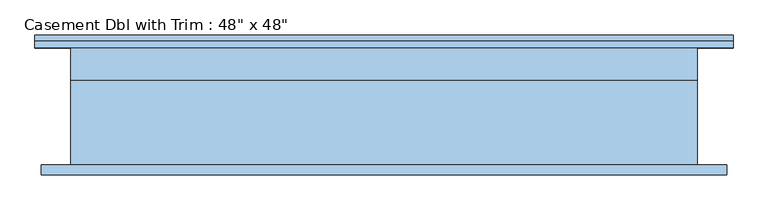
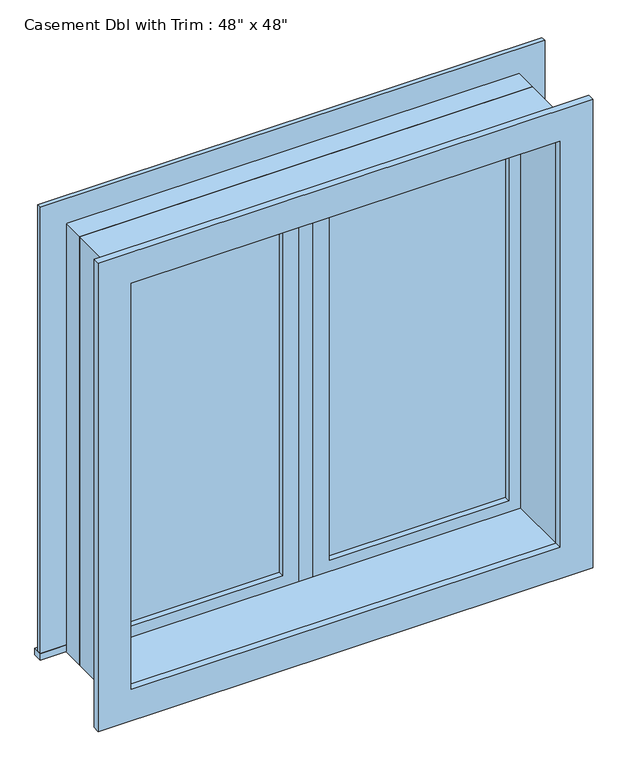
"""IFC4 building model written with IfcOpenShell, lengths in millimetres: window geometry."""

from ifc_helpers import new_model, si_unit, frame, origin, place, context, project, spatial, polyline, outline, extrude, source, transform, mapped, element, save


def window_534dcd48(model_context):
    return source(origin(), model_context, "Body", "SweptSolid", [
        extrude(outline(polyline([(63.5, 98.425), (546.1, 98.425), (546.1, 85.725), (63.5, 85.725), (63.5, 98.425)])), frame((0.0, 0.0, 977.9), z_axis=(0.0, 0.0, 1.0), x_axis=(1.0, 0.0, 0.0)), (0.0, 0.0, 1.0), 1092.2),
        extrude(outline(polyline([(2114.55, 19.05), (933.45, 19.05), (933.45, 590.55), (2114.55, 590.55), (2114.55, 19.05)]), holes=[polyline([(2070.1, 63.5), (2070.1, 546.1), (977.9, 546.1), (977.9, 63.5), (2070.1, 63.5)])]), frame((0.0, 69.85, 0.0), z_axis=(0.0, 1.0, 0.0), x_axis=(0.0, 0.0, 1.0)), (0.0, 0.0, 1.0), 44.45),
        extrude(outline(polyline([(19.05, 69.85), (-19.05, 69.85), (-19.05, 133.35), (19.05, 133.35), (19.05, 69.85)])), frame((0.0, 0.0, 933.45), z_axis=(0.0, 0.0, 1.0), x_axis=(1.0, 0.0, 0.0)), (0.0, 0.0, 1.0), 1181.1),
        extrude(outline(polyline([(-679.45, 158.75), (679.45, 158.75), (679.45, 133.35), (-679.45, 133.35), (-679.45, 158.75)])), frame((0.0, 0.0, 914.4), z_axis=(0.0, 0.0, 1.0), x_axis=(1.0, 0.0, 0.0)), (0.0, 0.0, 1.0), 19.05),
        extrude(outline(polyline([(2114.55, -590.55), (2114.55, 590.55), (933.45, 590.55), (933.45, 679.45), (2203.45, 679.45), (2203.45, -679.45), (933.45, -679.45), (933.45, -590.55), (2114.55, -590.55)])), frame((0.0, 133.35, 0.0), z_axis=(0.0, 1.0, 0.0), x_axis=(0.0, 0.0, 1.0)), (0.0, 0.0, 1.0), 12.7),
        extrude(outline(polyline([(2190.75, 666.75), (2190.75, -666.75), (857.25, -666.75), (857.25, 666.75), (2190.75, 666.75)]), holes=[polyline([(2101.85, 577.85), (946.15, 577.85), (946.15, -577.85), (2101.85, -577.85), (2101.85, 577.85)])]), frame((0.0, -114.3, 0.0), z_axis=(0.0, 1.0, 0.0), x_axis=(0.0, 0.0, 1.0)), (0.0, 0.0, 1.0), 19.05),
        extrude(outline(polyline([(-63.5, 85.725), (-546.1, 85.725), (-546.1, 98.425), (-63.5, 98.425), (-63.5, 85.725)])), frame((0.0, 0.0, 977.9), z_axis=(0.0, 0.0, 1.0), x_axis=(1.0, 0.0, 0.0)), (0.0, 0.0, 1.0), 1092.2),
        extrude(outline(polyline([(2114.55, -590.55), (933.45, -590.55), (933.45, -19.05), (2114.55, -19.05), (2114.55, -590.55)]), holes=[polyline([(2070.1, -546.1), (2070.1, -63.5), (977.9, -63.5), (977.9, -546.1), (2070.1, -546.1)])]), frame((0.0, 69.85, 0.0), z_axis=(0.0, 1.0, 0.0), x_axis=(0.0, 0.0, 1.0)), (0.0, 0.0, 1.0), 44.45),
        extrude(outline(polyline([(2133.6, -609.6), (914.4, -609.6), (914.4, 609.6), (2133.6, 609.6), (2133.6, -609.6)]), holes=[polyline([(2101.85, -577.85), (2101.85, 577.85), (946.15, 577.85), (946.15, -577.85), (2101.85, -577.85)])]), frame((0.0, -95.25, 0.0), z_axis=(0.0, 1.0, 0.0), x_axis=(0.0, 0.0, 1.0)), (0.0, 0.0, 1.0), 165.1),
        extrude(outline(polyline([(2133.6, 609.6), (2133.6, -609.6), (914.4, -609.6), (914.4, 609.6), (2133.6, 609.6)]), holes=[polyline([(2114.55, 590.55), (933.45, 590.55), (933.45, -590.55), (2114.55, -590.55), (2114.55, 590.55)])]), frame((0.0, 69.85, 0.0), z_axis=(0.0, 1.0, 0.0), x_axis=(0.0, 0.0, 1.0)), (0.0, 0.0, 1.0), 63.5),
    ])


if __name__ == "__main__":
    model = new_model("IFC4")
    model_context = context("Model", 3, world=origin())
    ifc_project = project(units=[si_unit("LENGTHUNIT", "METRE", prefix="MILLI")], contexts=[model_context])
    site = spatial("IfcSite", under=ifc_project)
    building = spatial("IfcBuilding", under=site)
    placement = place(None, origin())
    window_shape = window_534dcd48(model_context)
    element("IfcWindow", 1, ObjectType="Casement Dbl with Trim : 48\" x 48\"", at=placement, inside=building, context=model_context, shape_type="MappedRepresentation", body=[
        mapped(window_shape, transform((0.0, 0.0, 0.0), x_axis=(1.0, 0.0, 0.0), y_axis=(0.0, 1.0, 0.0), z_axis=(0.0, 0.0, 1.0))),
    ])
    save(model, "model.ifc")

# Revit data of these elements
# Type "Casement Dbl with Trim : 48\" x 48\""
#   Type Mark = "19"
#   Construction Type Id = "GSP4R"
#   Assembly Code = "B2020100"
#   Analytic Construction = "1/8 in Pilkington single glazing"
#   Visual Light Transmittance = 0.9
#   Solar Heat Gain Coefficient = 0.78
#   Heat Transfer Coefficient (U) = 0.6496 BTU/(h·ft²·°F)
#   Height = 4' - 0"
#   Default Sill Height = 3' - 0"
#   Trim Projection - Ext. = 0' - 0 1/2"
#   Trim Projection - Int. = 0' - 0 3/4"
#   Trim Width - Exterior = 0' - 3 1/2"
#   Trim Width - Interior = 0' - 3 1/2"
#   Width = 4' - 0"
#   Window Inset = 0' - 0 3/4"
#   Define Thermal Properties by = 1
#   Glass Pane Material = Glass
#   Sash Material = Sash
#   Trim Exterior Material = Trim
#   Trim Interior Material = Trim
#   Wall Closure = (empty or 0)
# Element 1 (IfcWindow, "Casement Dbl with Trim : 48\" x 48\"")
#   Materials on its faces: "Sash", "Trim", "Glass"
# Materials
#   "Glass": class "Glass", colour RGB 0 128 192, transparency 0.75, Description = "Soda Lime Glass", Cost = 0
#   "Sash": class "Wood", colour RGB 224 178 126, transparency 0
#   "Trim": class "Wood", colour RGB 224 178 126, transparency 0
